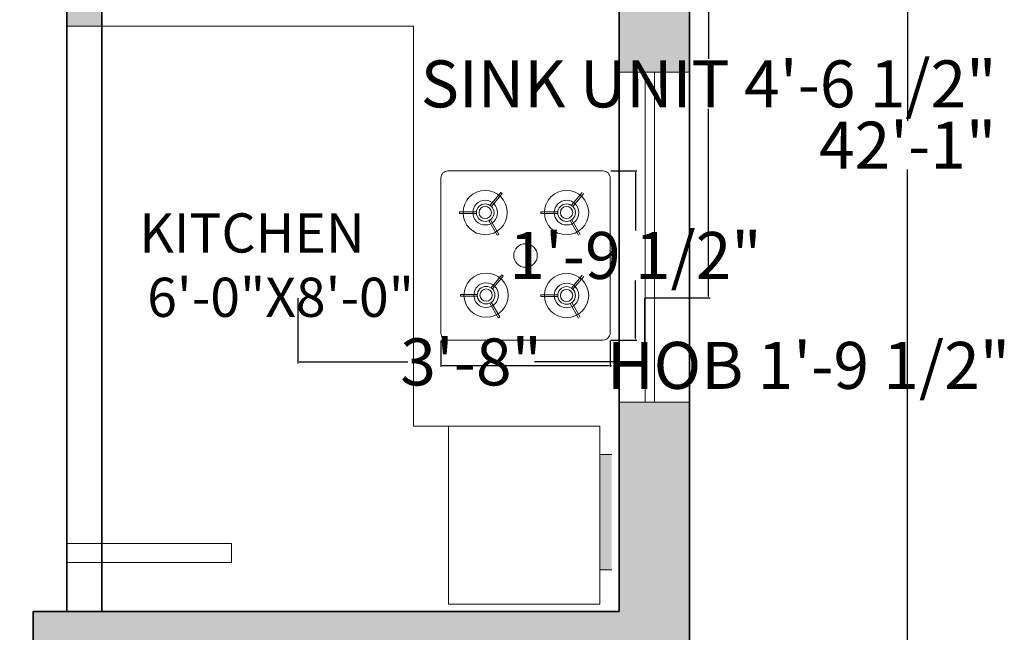
# Model space of a CAD drawing. Units: inches. Extents: x 143233372 to 143233714, y 112671713 to 112672292.
# Tile 4 of 7: x 143233571 to 143233696, y 112671935 to 112672013. Entities that reach past the tile are written whole.
import ezdxf

# ---------------------------------------------------------------- set-up
doc = ezdxf.new("R2010")
doc.units = ezdxf.units.IN
doc.header["$MEASUREMENT"] = 0
doc.layers.get('0').update_dxf_attribs({"color": 104})
for name, color, linetype, lineweight in [('A-ANNO-DIMS', 2, 'Continuous', 18), ('A-AREA-IDEN', 7, 'Continuous', 18), ('A-EQPM', 8, 'Continuous', 18), ('A-FLOR-CASE', 32, 'Continuous', 18), ('furniture', 23, 'Continuous', 18), ('walls', 7, 'Continuous', 35), ('windows', 4, 'Continuous', 18)]:
    doc.layers.add(name, color=color, linetype=linetype, lineweight=lineweight)
doc.layers.add('A-WALL-PATT', color=18, linetype='Continuous', lineweight=9, true_color=0x000000)
doc.styles.get("Standard").update_dxf_attribs({"font": 'arial.ttf'})
doc.dimstyles.get("Standard").update_dxf_attribs({"dimtxt": 6, "dimasz": 0.18, "dimexe": 0.18, "dimexo": 0.0625, "dimgap": 0.09, "dimtad": 0, "dimtih": 1, "dimtoh": 1, "dimzin": 0, "dimdsep": 46, "dimlunit": 3, "dimtxsty": 'Standard', "dimcen": 0.09, "dimadec": 0, "dimazin": 0, "dimtfac": 1, "dimtofl": 0, "dimtmove": 0, "dimatfit": 3, "dimfxl": 1, "dimtolj": 1, "dimtzin": 0, "dimarcsym": 0})

# ---------------------------------------------------------------- blocks, each defined once
blk = doc.blocks.new('4bstove')
at = {"layer": 'furniture'}
for p, q in [((1452.73, 1446.21), (1452.73, 1448.61)), ((1452.98, 1446.22), (1452.98, 1448.61)), ((1464.44, 1446.34), (1464.44, 1448.73)), ((1464.69, 1446.34), (1464.69, 1448.73)), ((1451.74, 1444.45), (1449.67, 1443.25)), ((1451.87, 1444.23), (1449.79, 1443.04)), ((1453.75, 1444.08), (1455.58, 1442.54)), ((1453.91, 1444.27), (1455.74, 1442.73)), ((1463.45, 1444.58), (1461.38, 1443.38)), ((1463.57, 1444.36), (1461.5, 1443.17)), ((1465.46, 1444.21), (1467.29, 1442.67)), ((1465.62, 1444.4), (1467.45, 1442.86)), ((1452.69, 1434.81), (1452.69, 1437.2)), ((1452.94, 1434.81), (1452.94, 1437.2)), ((1464.44, 1434.81), (1464.44, 1437.2)), ((1464.69, 1434.81), (1464.69, 1437.2)), ((1451.7, 1433.04), (1449.63, 1431.85)), ((1451.82, 1432.83), (1449.75, 1431.63)), ((1453.71, 1432.67), (1455.54, 1431.13)), ((1453.87, 1432.86), (1455.7, 1431.33)), ((1463.45, 1433.04), (1461.38, 1431.85)), ((1463.57, 1432.83), (1461.5, 1431.63)), ((1465.46, 1432.67), (1467.29, 1431.13)), ((1465.62, 1432.86), (1467.45, 1431.33))]:
    blk.add_line(p, q, dxfattribs=at)
for points in [[(1447.5, 1427.38), (1469.5, 1427.38, 0.414214), (1470.5, 1428.38), (1470.5, 1450.38, 0.414214), (1469.5, 1451.38), (1447.5, 1451.38, 0.414214), (1446.5, 1450.38), (1446.5, 1428.38, 0.414214)], [(1453.75, 1444.97, 1), (1452, 1444.97, 1)], [(1465.46, 1445.1, 1), (1463.71, 1445.1, 1)], [(1453.71, 1433.56, 1), (1451.96, 1433.56, 1)], [(1465.46, 1433.56, 1), (1463.71, 1433.56, 1)]]:
    blk.add_lwpolyline(points, format="xyb", close=True, dxfattribs=at)
for points in [[(1454.12, 1444.97, 1), (1451.62, 1444.97, 1), (1454.12, 1444.97, 1)], [(1465.83, 1445.1, 1), (1463.33, 1445.1, 1), (1465.83, 1445.1, 1)], [(1454.08, 1433.56, 1), (1451.58, 1433.56, 1), (1454.08, 1433.56, 1)], [(1465.83, 1433.56, 1), (1463.33, 1433.56, 1), (1465.83, 1433.56, 1)]]:
    blk.add_lwpolyline(points, format="xyb", dxfattribs=at)
for centre, radius in [((1452.87, 1444.97), 3.14), ((1464.58, 1445.1), 3.14), ((1452.87, 1444.97), 1.75), ((1464.58, 1445.1), 1.75), ((1458.5, 1439.38), 1.67), ((1452.83, 1433.56), 3.14), ((1464.58, 1433.56), 3.14), ((1452.83, 1433.56), 1.75), ((1464.58, 1433.56), 1.75)]:
    blk.add_circle(centre, radius, dxfattribs=at)
for centre, start, end in [((1452.87, 1444.97), 88.2645, 92.2039), ((1464.58, 1445.1), 88.2645, 92.2039), ((1452.87, 1444.97), 208.188, 212.1274), ((1452.87, 1444.97), 318.1018, 322.0412), ((1464.58, 1445.1), 208.188, 212.1274), ((1464.58, 1445.1), 318.1018, 322.0412), ((1452.83, 1433.56), 88.2645, 92.2039), ((1464.58, 1433.56), 88.2645, 92.2039)]:
    blk.add_arc(centre, 3.64, start, end, dxfattribs=at)
blk = doc.blocks.new('stove')
at = {"layer": 'furniture', "xscale": 0.9, "yscale": 0.9, "zscale": 0.9, "rotation": 89.99999999999999}
blk.add_blockref('4bstove', (1295.44, -1312.65), dxfattribs=at)
blk = doc.blocks.new('SASH-42IN')
for p, q in [((0, 1.17), (42.12, 1.17)), ((42.12, 0), (0, 0)), ((42.12, 1.17), (42.12, 0))]:
    blk.add_line(p, q)
blk = doc.blocks.new('*D57')
at = {"layer": 'A-ANNO-DIMS', "color": 0, "lineweight": -2, "transparency": 16777216}
for p, q in [((143233650.58, 112672031.88), (143233658.89, 112672031.88)), ((143233658.71, 112672031.7), (143233658.71, 112672007.75)), ((143233658.71, 112671977.41), (143233658.71, 112672001.36)), ((143233650.58, 112671977.23), (143233658.89, 112671977.23))]:
    blk.add_line(p, q, dxfattribs=at)
at = {"layer": 'A-ANNO-DIMS', "color": 0, "transparency": 16777216}
for points in [[(143233658.68, 112672031.7), (143233658.74, 112672031.7), (143233658.71, 112672031.88)], [(143233658.68, 112671977.41), (143233658.74, 112671977.41), (143233658.71, 112671977.23)]]:
    blk.add_solid(points, dxfattribs=at)
at = {"layer": 'Defpoints', "color": 0, "transparency": 16777216}
for p in [(143233650.52, 112672031.88), (143233650.52, 112671977.23), (143233658.71, 112671977.23)]:
    blk.add_point(p, dxfattribs=at)
at = {"layer": 'A-ANNO-DIMS', "color": 0, "transparency": 16777216, "insert": (143233658.71, 112672004.55), "char_height": 6, "attachment_point": 5}
blk.add_mtext('\\A1;SINK UNIT 4\'-6 1/2"', dxfattribs=at)
blk = doc.blocks.new('*D58')
at = {"layer": 'A-ANNO-DIMS', "color": 0, "lineweight": -2, "transparency": 16777216}
for p, q in [((143233606.29, 112671977.17), (143233606.29, 112671968.86)), ((143233650.52, 112671977.17), (143233650.52, 112671968.86)), ((143233606.47, 112671969.04), (143233620.34, 112671969.04)), ((143233650.34, 112671969.04), (143233636.47, 112671969.04))]:
    blk.add_line(p, q, dxfattribs=at)
at = {"layer": 'A-ANNO-DIMS', "color": 0, "transparency": 16777216}
for points in [[(143233606.47, 112671969.07), (143233606.47, 112671969.01), (143233606.29, 112671969.04)], [(143233650.34, 112671969.07), (143233650.34, 112671969.01), (143233650.52, 112671969.04)]]:
    blk.add_solid(points, dxfattribs=at)
at = {"layer": 'Defpoints', "color": 0, "transparency": 16777216}
for p in [(143233606.29, 112671977.23), (143233650.52, 112671977.23), (143233606.29, 112671969.04)]:
    blk.add_point(p, dxfattribs=at)
at = {"layer": 'A-ANNO-DIMS', "color": 0, "transparency": 16777216, "insert": (143233628.4, 112671969.04), "char_height": 6, "attachment_point": 5}
blk.add_mtext('\\A1;3\'-8"', dxfattribs=at)
blk = doc.blocks.new('*D59')
at = {"layer": 'A-ANNO-DIMS', "color": 0, "lineweight": -2, "transparency": 16777216}
for p, q in [((143233624.54, 112671971.77), (143233624.54, 112671968.42)), ((143233646.14, 112671971.77), (143233646.14, 112671968.42)), ((143233624.72, 112671968.6), (143233645.96, 112671968.6)), ((143233646.14, 112671968.6), (143233646.32, 112671968.6))]:
    blk.add_line(p, q, dxfattribs=at)
at = {"layer": 'A-ANNO-DIMS', "color": 0, "transparency": 16777216}
for points in [[(143233624.72, 112671968.63), (143233624.72, 112671968.57), (143233624.54, 112671968.6)], [(143233645.96, 112671968.63), (143233645.96, 112671968.57), (143233646.14, 112671968.6)]]:
    blk.add_solid(points, dxfattribs=at)
at = {"layer": 'Defpoints', "color": 0, "transparency": 16777216}
for p in [(143233624.54, 112671971.84), (143233646.14, 112671971.84), (143233646.14, 112671968.6)]:
    blk.add_point(p, dxfattribs=at)
at = {"layer": 'A-ANNO-DIMS', "color": 0, "transparency": 16777216, "insert": (143233671.46, 112671968.6), "char_height": 6, "attachment_point": 5}
blk.add_mtext('\\A1;HOB 1\'-9 1/2"', dxfattribs=at)
blk = doc.blocks.new('*D60')
at = {"layer": 'A-ANNO-DIMS', "color": 0, "lineweight": -2, "transparency": 16777216}
for p, q in [((143233646.21, 112671993.44), (143233649.56, 112671993.44)), ((143233649.38, 112671993.26), (143233649.38, 112671985.83)), ((143233649.38, 112671972.02), (143233649.38, 112671979.44)), ((143233646.21, 112671971.84), (143233649.56, 112671971.84))]:
    blk.add_line(p, q, dxfattribs=at)
at = {"layer": 'A-ANNO-DIMS', "color": 0, "transparency": 16777216}
for points in [[(143233649.35, 112671993.26), (143233649.41, 112671993.26), (143233649.38, 112671993.44)], [(143233649.35, 112671972.02), (143233649.41, 112671972.02), (143233649.38, 112671971.84)]]:
    blk.add_solid(points, dxfattribs=at)
at = {"layer": 'Defpoints', "color": 0, "transparency": 16777216}
for p in [(143233646.14, 112671993.44), (143233649.38, 112671993.44), (143233646.14, 112671971.84)]:
    blk.add_point(p, dxfattribs=at)
at = {"layer": 'A-ANNO-DIMS', "color": 0, "transparency": 16777216, "insert": (143233649.38, 112671982.64), "char_height": 6, "attachment_point": 5}
blk.add_mtext('\\A1;1\'-9 1/2"', dxfattribs=at)
blk = doc.blocks.new('*D63')
at = {"layer": 'A-ANNO-DIMS', "color": 0, "lineweight": -2, "transparency": 16777216}
for p, q in [((143233656.35, 112672249.18), (143233684.29, 112672249.18)), ((143233684.11, 112672249), (143233684.11, 112671999.82)), ((143233684.11, 112671744.43), (143233684.11, 112671993.61)), ((143233656.35, 112671744.25), (143233684.29, 112671744.25))]:
    blk.add_line(p, q, dxfattribs=at)
at = {"layer": 'A-ANNO-DIMS', "color": 0, "transparency": 16777216}
for points in [[(143233684.08, 112672249), (143233684.14, 112672249), (143233684.11, 112672249.18)], [(143233684.08, 112671744.43), (143233684.14, 112671744.43), (143233684.11, 112671744.25)]]:
    blk.add_solid(points, dxfattribs=at)
at = {"layer": 'Defpoints', "color": 0, "transparency": 16777216}
for p in [(143233656.28, 112672249.18), (143233656.28, 112671744.25), (143233684.11, 112671744.25)]:
    blk.add_point(p, dxfattribs=at)
at = {"layer": 'A-ANNO-DIMS', "color": 0, "transparency": 16777216, "insert": (143233684.11, 112671996.72), "char_height": 6, "attachment_point": 5}
blk.add_mtext('\\A1;42\'-1"', dxfattribs=at)

msp = doc.modelspace()

# ---------------------------------------------------------------- hatches: boundary and pattern name
at = {"layer": 'A-EQPM'}
h = msp.add_hatch(color=256, dxfattribs=at)
h.dxf.hatch_style = 1
h.paths.add_polyline_path([(143233646.343, 112671957.226), (143233644.828, 112671957.226), (143233644.828, 112671942.475), (143233646.343, 112671942.475)])
at = {"layer": 'A-WALL-PATT'}
h = msp.add_hatch(color=256, dxfattribs=at)
h.dxf.hatch_style = 1
h.paths.add_polyline_path([(143233425.285, 112671820.328), (143233416.222, 112671820.328), (143233416.222, 112671767.682), (143233464.805, 112671767.682), (143233464.805, 112671776.682), (143233425.285, 112671776.682)])
h.paths.add_polyline_path([(143233425.285, 112672055.48), (143233416.285, 112672055.48), (143233416.285, 112671984.159), (143233425.285, 112671984.159)])
h.paths.add_polyline_path([(143233656.285, 112671963.912), (143233647.285, 112671963.912), (143233647.285, 112671848.682), (143233647.285, 112671839.682), (143233656.285, 112671839.682), (143233656.285, 112671889.182)])
h.paths.add_polyline_path([(143233425.285, 112672097.332), (143233425.285, 112672097.332), (143233425.285, 112672108.216), (143233425.285, 112672240.182), (143233451.497, 112672240.182), (143233451.497, 112672249.182), (143233416.285, 112672249.182), (143233416.285, 112672079.453), (143233420.069, 112672079.453), (143233425.285, 112672079.453)])
h.paths.add_polyline_path([(143233576.214, 112672249.182), (143233493.616, 112672249.182), (143233493.616, 112672240.182), (143233576.214, 112672240.182)])
h.paths.add_polyline_path([(143233425.285, 112671942.039), (143233416.285, 112671942.039), (143233416.285, 112671889.182), (143233416.271, 112671862.447), (143233425.285, 112671862.447), (143233425.285, 112671896.682), (143233518.63, 112671896.682, -0.0122006), (143233518.603, 112671897.787), (143233518.603, 112671901.182), (143233425.285, 112671901.182)])
h = msp.add_hatch(color=256, dxfattribs=at)
h.dxf.hatch_style = 1
h.paths.add_polyline_path([(143233656.285, 112672249.182), (143233647.285, 112672249.182), (143233647.285, 112672240.182), (143233656.285, 112672240.182)])
h.paths.add_polyline_path([(143233647.285, 112672249.182), (143233618.333, 112672249.182), (143233618.333, 112672240.182), (143233647.285, 112672240.182)])
h.paths.add_polyline_path([(143233656.285, 112672240.182), (143233647.285, 112672240.182), (143233647.285, 112672096.182), (143233656.285, 112672096.182)])
h.paths.add_polyline_path([(143233656.285, 112672096.182), (143233647.285, 112672096.182), (143233647.285, 112672091.682), (143233656.285, 112672091.682)])
h.paths.add_polyline_path([(143233647.285, 112672096.182), (143233581.998, 112672096.182), (143233581.998, 112672091.682), (143233647.285, 112672091.682)])
h.paths.add_polyline_path([(143233656.285, 112672091.682), (143233647.285, 112672091.682), (143233647.285, 112672037.682), (143233656.285, 112672037.682)])
h.paths.add_polyline_path([(143233656.285, 112672037.682), (143233647.285, 112672037.682), (143233647.285, 112672033.182), (143233656.285, 112672033.182)])
h.paths.add_polyline_path([(143233656.285, 112672033.182), (143233647.285, 112672033.182), (143233647.285, 112672006.032), (143233656.285, 112672006.032)])
h = msp.add_hatch(color=256, dxfattribs=at)
h.dxf.hatch_style = 1
h.paths.add_polyline_path([(143233549.785, 112671901.182), (143233541.241, 112671901.182), (143233541.241, 112671897.787), (143233541.241, 112671896.682), (143233545.285, 112671896.682), (143233545.285, 112671848.682), (143233549.785, 112671848.682)])
h.paths.add_polyline_path([(143233581.285, 112672033.182), (143233576.785, 112672033.182), (143233576.785, 112672011.912), (143233581.285, 112672011.912)])
h = msp.add_hatch(color=256, dxfattribs=at)
h.dxf.hatch_style = 1
h.paths.add_polyline_path([(143233647.285, 112671937.182), (143233572.511, 112671937.182), (143233572.511, 112671932.682), (143233647.285, 112671932.682)])

# ---------------------------------------------------------------- linework, layer by layer
at = {"layer": 'A-EQPM'}
for p, q in [((143233625.531, 112671938.127), (143233625.531, 112671960.851)), ((143233625.531, 112671960.851), (143233644.828, 112671960.851)), ((143233644.828, 112671960.851), (143233644.828, 112671938.127)), ((143233646.347, 112671957.226), (143233644.828, 112671957.226)), ((143233644.828, 112671942.475), (143233646.347, 112671942.475)), ((143233644.828, 112671938.127), (143233625.531, 112671938.127))]:
    msp.add_line(p, q, dxfattribs=at)
at = {"layer": 'A-FLOR-CASE'}
for p, q in [((143233576.785, 112672011.912), (143233621.037, 112672011.912)), ((143233581.285, 112672011.912), (143233581.285, 112672011.912)), ((143233621.037, 112672011.912), (143233621.037, 112671961.61)), ((143233621.037, 112671961.61), (143233621.037, 112671960.851)), ((143233621.037, 112671960.851), (143233625.531, 112671960.851)), ((143233576.785, 112671945.841), (143233597.802, 112671945.841)), ((143233597.802, 112671945.841), (143233597.802, 112671943.41)), ((143233597.802, 112671943.41), (143233576.785, 112671943.41))]:
    msp.add_line(p, q, dxfattribs=at)
at = {"layer": 'walls'}
for p, q in [((143233656.285, 112672249.182), (143233656.285, 112671889.182)), ((143233576.785, 112671937.182), (143233576.785, 112672037.682)), ((143233581.285, 112672037.682), (143233581.285, 112671937.182)), ((143233647.285, 112672037.682), (143233647.285, 112671937.182)), ((143233576.785, 112671937.182), (143233576.785, 112672033.182)), ((143233581.285, 112671937.182), (143233581.285, 112672033.182)), ((143233572.511, 112671937.182), (143233647.285, 112671937.182)), ((143233572.511, 112671937.182), (143233572.511, 112671932.682))]:
    msp.add_line(p, q, dxfattribs=at)
at = {"layer": 'windows'}
for p, q in [((143233656.285, 112672006.032), (143233647.285, 112672006.032)), ((143233647.285, 112671963.912), (143233656.285, 112671963.912))]:
    msp.add_line(p, q, dxfattribs=at)

# ---------------------------------------------------------------- block references
at = {"layer": 'A-EQPM'}
msp.add_blockref('stove', (143233635.343, 112671982.635), dxfattribs=at)
at = {"layer": 'windows', "rotation": 89.99999996834183}
msp.add_blockref('SASH-42IN', (143233651.785, 112671963.913), dxfattribs=at)

# ---------------------------------------------------------------- texts
at = {"layer": 'A-AREA-IDEN'}
for s, p in [('KITCHEN', (143233586.045, 112671983.012)), ('6\'-0"X8\'-0"', (143233587.063, 112671974.798))]:
    msp.add_text(s, height=5, dxfattribs=at).set_placement(p)

# ---------------------------------------------------------------- dimensions: what is measured, and where the dimension line sits
at = {"layer": 'A-ANNO-DIMS'}
for base, p1, p2, angle, picture, middle in [((143233684.111, 112671744.249), (143233656.285, 112672249.182), (143233656.285, 112671744.249), 90, '*D63', (143233684.111, 112671996.716)), ((143233649.383, 112671993.435), (143233646.143, 112671971.835), (143233646.143, 112671993.435), 90, '*D60', (143233649.383, 112671982.635)), ((143233606.288, 112671969.036), (143233650.518, 112671977.233), (143233606.288, 112671977.233), 180, '*D58', (143233628.403, 112671969.036))]:
    dim = msp.add_linear_dim(base=base, p1=p1, p2=p2, angle=angle, dimstyle='Standard', override={"dimdec": 1, "dimlfac": 1, "dimrnd": 0, "dimzin": 1, "dimdsep": 46, "dimlunit": 4, "dimfrac": 2}, dxfattribs=at)
    dim.commit()
    dim.dimension.update_dxf_attribs({"geometry": picture, "text_midpoint": middle})
dim = msp.add_linear_dim(base=(143233658.714, 112671977.233), p1=(143233650.518, 112672031.875), p2=(143233650.518, 112671977.233), angle=270, text='SINK UNIT <>', dimstyle='Standard', override={"dimdec": 1, "dimlfac": 1, "dimrnd": 0, "dimzin": 1, "dimdsep": 46, "dimlunit": 4, "dimfrac": 2}, dxfattribs=at)
dim.commit()
dim.dimension.update_dxf_attribs({"geometry": '*D57', "text_midpoint": (143233658.714, 112672004.554)})
dim = msp.add_linear_dim(base=(143233646.143, 112671968.595), p1=(143233624.543, 112671971.835), p2=(143233646.143, 112671971.835), text='HOB <>', dimstyle='Standard', override={"dimdec": 1, "dimlfac": 1, "dimrnd": 0, "dimzin": 1, "dimdsep": 46, "dimlunit": 4, "dimfrac": 2}, dxfattribs=at)
dim.commit()
dim.dimension.update_dxf_attribs({"geometry": '*D59', "text_midpoint": (143233671.463, 112671968.595)})

doc.saveas('drawing.dxf')
